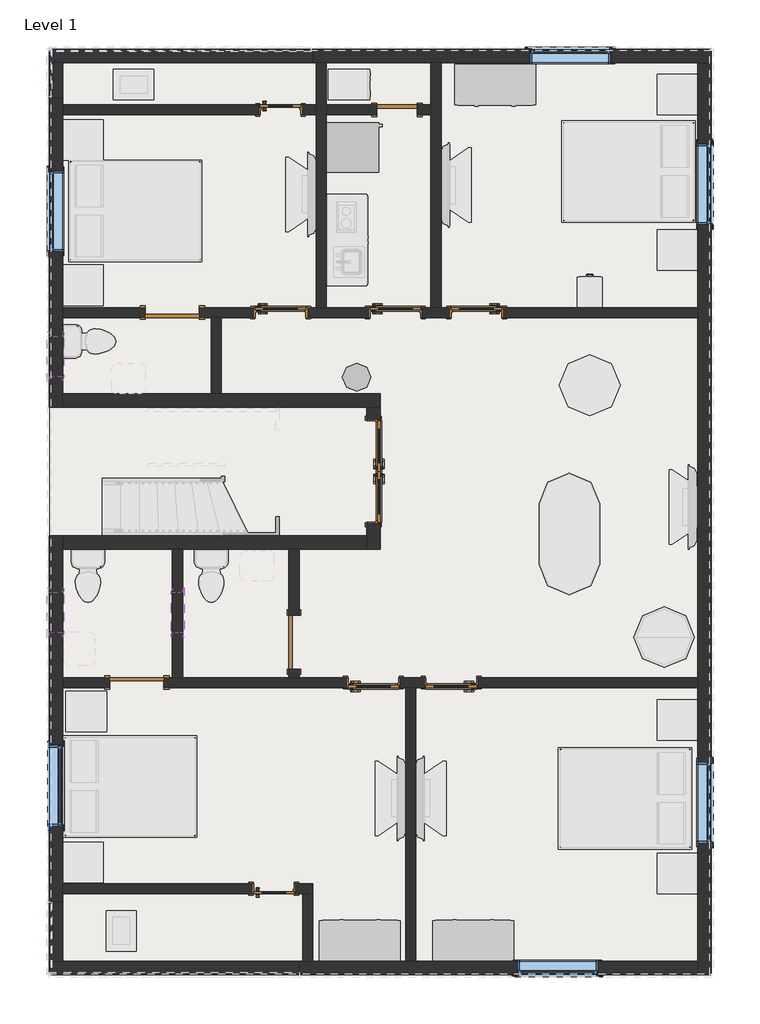
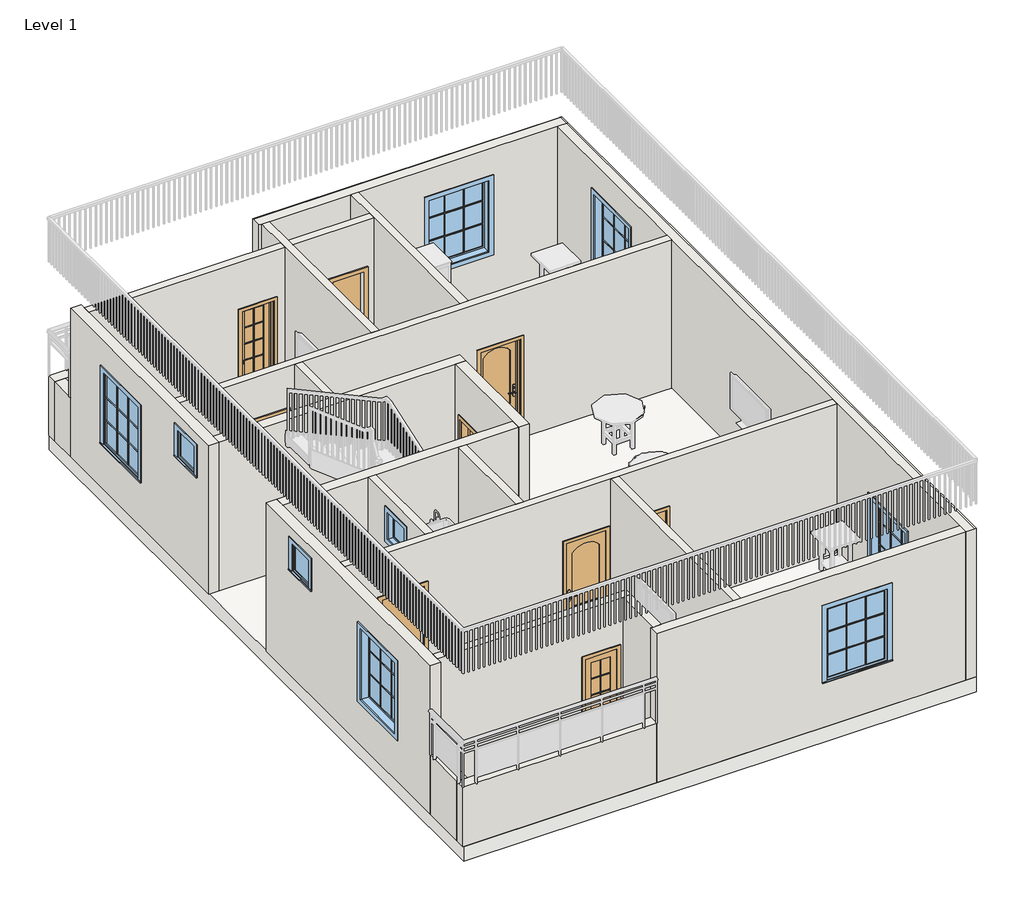
# One storey, part 1 of 7: 24 walls, 12 doors, 9 windows, 1 slab.
"""IFC4 building model written with IfcOpenShell, lengths in millimetres."""

from ifc_helpers import new_model, si_unit, frame, origin, origin_with_axes, place, context, project, spatial, polyline, outline, extrude, faceted_brep, transform, mapped, element, save
from components import door_14b9be53, door_4b146b56, door_b03bd389, door_921d1c85, door_6d64ae12, door_58dae0ba, door_bb092f7c, door_377e7377, window_99fc0ff6, window_2b070d82, window_e41d21a6, window_3d781103

model = new_model("IFC4")

# Units and contexts
model_context = context("Model", 3, world=origin())
ifc_project = project(units=[si_unit("LENGTHUNIT", "METRE", prefix="MILLI")], contexts=[model_context])

# Site, building, storey
site = spatial("IfcSite", under=ifc_project)
building = spatial("IfcBuilding", under=site)
storey = spatial("IfcBuildingStorey", under=building, Name="Level 1", Elevation=0.0)

# Doors
placement = place(None, origin())
door_shape = door_14b9be53(model_context)
element("IfcDoor", 1, ObjectType="30\" x 80\"", at=placement, inside=storey, context=model_context, shape_type="MappedRepresentation", body=[
    mapped(door_shape, transform((-2054.08475, 8491.4589473, 0.0), x_axis=(1.0, 0.0, 0.0), y_axis=(0.0, 1.0, 0.0), z_axis=(0.0, 0.0, 1.0))),
])
element("IfcDoor", 2, ObjectType="30\" x 80\"", at=placement, inside=storey, context=model_context, shape_type="MappedRepresentation", body=[
    mapped(door_shape, transform((-3603.48475, 2922.5089473, 0.0), x_axis=(-1.0, 0.0, 0.0), y_axis=(0.0, -1.0, 0.0), z_axis=(0.0, 0.0, 1.0))),
])
door_2_shape = door_4b146b56(model_context)
element("IfcDoor", 3, ObjectType="30\" x 80\"", at=placement, inside=storey, context=model_context, shape_type="MappedRepresentation", body=[
    mapped(door_2_shape, transform((-2435.08475, 2922.5089473, 0.0), x_axis=(1.0, 0.0, 0.0), y_axis=(0.0, 1.0, 0.0), z_axis=(0.0, 0.0, 1.0))),
])
element("IfcDoor", 4, ObjectType="30\" x 80\"", at=placement, inside=storey, context=model_context, shape_type="MappedRepresentation", body=[
    mapped(door_2_shape, transform((-5000.48475, 8491.4589473, 0.0), x_axis=(-1.0, 0.0, 0.0), y_axis=(0.0, -1.0, 0.0), z_axis=(0.0, 0.0, 1.0))),
])
element("IfcDoor", 5, ObjectType="30\" x 80\"", at=placement, inside=storey, context=model_context, shape_type="MappedRepresentation", body=[
    mapped(door_2_shape, transform((-3273.28475, 8491.4589473, 0.0), x_axis=(-1.0, 0.0, 0.0), y_axis=(0.0, -1.0, 0.0), z_axis=(0.0, 0.0, 1.0))),
])
door_3_shape = door_b03bd389(model_context)
element("IfcDoor", 6, ObjectType="Door-Exterior-Double-Full Glass-Wood_Clad : 60\" x 80\"", at=placement, inside=storey, context=model_context, shape_type="MappedRepresentation", body=[
    mapped(door_3_shape, transform((-3600.30975, 6100.6839473, 0.0), x_axis=(0.0, -1.0, 0.0), y_axis=(1.0, 0.0, 0.0), z_axis=(0.0, 0.0, 1.0))),
])
door_4_shape = door_921d1c85(model_context)
element("IfcDoor", 7, ObjectType="Door-Interior-Single-Full Glass-Wood : 24\" x 80\"", at=placement, inside=storey, context=model_context, shape_type="MappedRepresentation", body=[
    mapped(door_4_shape, transform((-5000.48475, 11539.4589473, 0.0), x_axis=(1.0, 0.0, 0.0), y_axis=(0.0, 1.0, 0.0), z_axis=(0.0, 0.0, 1.0))),
])
door_5_shape = door_6d64ae12(model_context)
element("IfcDoor", 8, ObjectType="Door-Interior-Single-Full Glass-Wood : 24\" x 80\"", at=placement, inside=storey, context=model_context, shape_type="MappedRepresentation", body=[
    mapped(door_5_shape, transform((-5102.08475, -176.2910527, 0.0), x_axis=(1.0, 0.0, 0.0), y_axis=(0.0, 1.0, 0.0), z_axis=(0.0, 0.0, 1.0))),
])
door_6_shape = door_58dae0ba(model_context)
element("IfcDoor", 9, ObjectType="Single-Flush : 24\" x 80\"", at=placement, inside=storey, context=model_context, shape_type="MappedRepresentation", body=[
    mapped(door_6_shape, transform((-3247.88475, 11536.2839473, 0.0), x_axis=(1.0, 0.0, 0.0), y_axis=(0.0, 1.0, 0.0), z_axis=(0.0, 0.0, 1.0))),
])
door_7_shape = door_bb092f7c(model_context)
element("IfcDoor", 10, ObjectType="Single-Flush : 32\" x 84\"", at=placement, inside=storey, context=model_context, shape_type="MappedRepresentation", body=[
    mapped(door_7_shape, transform((-4797.28475, 3535.2839473, 0.0), x_axis=(0.0, -1.0, 0.0), y_axis=(1.0, 0.0, 0.0), z_axis=(0.0, 0.0, 1.0))),
])
element("IfcDoor", 11, ObjectType="Single-Flush : 32\" x 84\"", at=placement, inside=storey, context=model_context, shape_type="MappedRepresentation", body=[
    mapped(door_7_shape, transform((-6626.08475, 8488.2839473, 0.0), x_axis=(1.0, 0.0, 0.0), y_axis=(0.0, 1.0, 0.0), z_axis=(0.0, 0.0, 1.0))),
])
door_8_shape = door_377e7377(model_context)
element("IfcDoor", 12, ObjectType="Single-Flush : 32\" x 84\"", at=placement, inside=storey, context=model_context, shape_type="MappedRepresentation", body=[
    mapped(door_8_shape, transform((-7159.48475, 2925.6839473, 0.0), x_axis=(1.0, 0.0, 0.0), y_axis=(0.0, 1.0, 0.0), z_axis=(0.0, 0.0, 1.0))),
])

# Slab
element("IfcSlab", 13, ObjectType="Generic - 12\"", at=placement, inside=storey, context=model_context, shape_type="SweptSolid", body=[
    extrude(outline(polyline([(-8467.58475, 12450.6839473), (1476.51525, 12450.6839473), (1476.51525, -1468.5160527), (-8467.58475, -1468.5160527), (-8467.58475, 12450.6839473)])), frame((0.0, 0.0, -304.8), z_axis=(0.0, 0.0, 1.0), x_axis=(1.0, 0.0, 0.0)), (0.0, 0.0, 1.0), 304.8),
])

# Walls
element("IfcWall", 14, ObjectType="Generic - 8\"", at=placement, inside=storey, context=model_context, shape_type="Brep", body=[
    faceted_brep([(-8480.28475, 12247.4839473, 0.0), (-8277.08475, 12247.4839473, 0.0), (-4517.88475, 12247.4839473, 0.0), (-4517.88475, 12247.4839473, 1219.2), (-8277.08475, 12247.4839473, 1219.2), (-8480.28475, 12247.4839473, 1219.2), (-8480.28475, 12450.6839473, 0.0), (-8480.28475, 12450.6839473, 1219.2), (-4517.88475, 12450.6839473, 1219.2), (-4517.88475, 12450.6839473, 0.0)], [[[0, 1, 2, 3, 4, 5]], [[6, 7, 8, 9]], [[2, 1, 0, 6, 9]], [[3, 2, 9, 8]], [[5, 4, 3, 8, 7]], [[0, 5, 7, 6]]]),
])
element("IfcWall", 15, ObjectType="Generic - 8\"", at=placement, inside=storey, context=model_context, shape_type="Brep", body=[
    faceted_brep([(1273.31525, 12247.4839473, 0.0), (1273.31525, 8564.4839473, 0.0), (1273.31525, 8412.0839473, 0.0), (1273.31525, 3001.8839473, 0.0), (1273.31525, 2849.4839473, 0.0), (1273.31525, -1265.3160527, 0.0), (1273.31525, -1468.5160527, 0.0), (1273.31525, -1468.5160527, 3048.0), (1273.31525, -1265.3160527, 3048.0), (1273.31525, 2849.4839473, 3048.0), (1273.31525, 3001.8839473, 3048.0), (1273.31525, 8412.0839473, 3048.0), (1273.31525, 8564.4839473, 3048.0), (1273.31525, 12247.4839473, 3048.0), (1273.31525, 512.6839473, 1828.8), (1273.31525, 512.6839473, 304.8), (1273.31525, 1731.8839473, 304.8), (1273.31525, 1731.8839473, 1828.8), (1273.31525, 9809.0839473, 2438.4), (1273.31525, 9809.0839473, 914.4), (1273.31525, 11028.2839473, 914.4), (1273.31525, 11028.2839473, 2438.4), (1476.51525, 12247.4839473, 0.0), (1476.51525, 12247.4839473, 3048.0), (1476.51525, -1468.5160527, 3048.0), (1476.51525, -1468.5160527, 0.0), (1476.51525, 512.6839473, 1828.8), (1476.51525, 1731.8839473, 1828.8), (1476.51525, 1731.8839473, 304.8), (1476.51525, 512.6839473, 304.8), (1476.51525, 9809.0839473, 2438.4), (1476.51525, 11028.2839473, 2438.4), (1476.51525, 11028.2839473, 914.4), (1476.51525, 9809.0839473, 914.4), (1451.11525, 12247.4839473, 3048.0), (1451.11525, -1468.5160527, 3048.0)], [[[0, 1, 2, 3, 4, 5, 6, 7, 8, 9, 10, 11, 12, 13], [14, 15, 16, 17], [18, 19, 20, 21]], [[22, 23, 24, 25], [26, 27, 28, 29], [30, 31, 32, 33]], [[6, 5, 4, 3, 2, 1, 0, 22, 25]], [[0, 13, 34, 23, 22]], [[7, 6, 25, 24, 35]], [[35, 24, 23, 34]], [[13, 12, 11, 10, 9, 8, 7, 35, 34]], [[15, 14, 26, 29]], [[16, 15, 29, 28]], [[17, 16, 28, 27]], [[14, 17, 27, 26]], [[19, 18, 30, 33]], [[20, 19, 33, 32]], [[21, 20, 32, 31]], [[18, 21, 31, 30]]]),
])
element("IfcWall", 16, ObjectType="Generic - 8\"", at=placement, inside=storey, context=model_context, shape_type="Brep", body=[
    faceted_brep([(1273.31525, -1265.3160527, 0.0), (-2968.48475, -1265.3160527, 0.0), (-3120.88475, -1265.3160527, 0.0), (-4517.88475, -1265.3160527, 0.0), (-4670.28475, -1265.3160527, 0.0), (-4721.08475, -1265.3160527, 0.0), (-4721.08475, -1265.3160527, 1219.2), (-4721.08475, -1265.3160527, 3048.0), (-4670.28475, -1265.3160527, 3048.0), (-4517.88475, -1265.3160527, 3048.0), (-3120.88475, -1265.3160527, 3048.0), (-2968.48475, -1265.3160527, 3048.0), (1273.31525, -1265.3160527, 3048.0), (-1444.48475, -1265.3160527, 2438.4), (-1444.48475, -1265.3160527, 914.4), (-225.28475, -1265.3160527, 914.4), (-225.28475, -1265.3160527, 2438.4), (1273.31525, -1468.5160527, 0.0), (1273.31525, -1468.5160527, 3048.0), (-4721.08475, -1468.5160527, 3048.0), (-4721.08475, -1468.5160527, 1219.2), (-4721.08475, -1468.5160527, 0.0), (-1444.48475, -1468.5160527, 2438.4), (-225.28475, -1468.5160527, 2438.4), (-225.28475, -1468.5160527, 914.4), (-1444.48475, -1468.5160527, 914.4)], [[[0, 1, 2, 3, 4, 5, 6, 7, 8, 9, 10, 11, 12], [13, 14, 15, 16]], [[17, 18, 19, 20, 21], [22, 23, 24, 25]], [[5, 4, 3, 2, 1, 0, 17, 21]], [[7, 6, 5, 21, 20, 19]], [[0, 12, 18, 17]], [[12, 11, 10, 9, 8, 7, 19, 18]], [[14, 13, 22, 25]], [[15, 14, 25, 24]], [[16, 15, 24, 23]], [[13, 16, 23, 22]]]),
])
element("IfcWall", 17, ObjectType="Generic - 8\"", at=placement, inside=storey, context=model_context, shape_type="SweptSolid", body=[
    extrude(outline(polyline([(-8277.08475, -376.3160527), (-8277.08475, -1265.3160527), (-8480.28475, -1265.3160527), (-8480.28475, -376.3160527), (-8277.08475, -376.3160527)])), origin_with_axes(), (0.0, 0.0, 1.0), 1219.2),
])
element("IfcWall", 18, ObjectType="Generic - 8\"", at=placement, inside=storey, context=model_context, shape_type="Brep", body=[
    faceted_brep([(-8277.08475, 7065.8839473, 0.0), (-3705.08475, 7065.8839473, 0.0), (-3501.88475, 7065.8839473, 0.0), (-3501.88475, 7065.8839473, 3048.0), (-3705.08475, 7065.8839473, 3048.0), (-6905.48475, 7065.8839473, 3048.0), (-8277.08475, 7065.8839473, 3048.0), (-8277.08475, 7269.0839473, 0.0), (-8277.08475, 7269.0839473, 3048.0), (-6041.88475, 7269.0839473, 3048.0), (-5889.48475, 7269.0839473, 3048.0), (-3501.88475, 7269.0839473, 3048.0), (-3501.88475, 7269.0839473, 0.0), (-5889.48475, 7269.0839473, 0.0), (-6041.88475, 7269.0839473, 0.0)], [[[0, 1, 2, 3, 4, 5, 6]], [[7, 8, 9, 10, 11, 12, 13, 14]], [[2, 1, 0, 7, 14, 13, 12]], [[3, 2, 12, 11]], [[0, 6, 8, 7]], [[6, 5, 4, 3, 11, 10, 9, 8]]]),
])
element("IfcWall", 19, ObjectType="Generic - 8\"", at=placement, inside=storey, context=model_context, shape_type="Brep", body=[
    faceted_brep([(-3705.08475, 7065.8839473, 3048.0), (-3705.08475, 7065.8839473, 0.0), (-3705.08475, 6888.0839473, 0.0), (-3705.08475, 6888.0839473, 2057.4), (-3705.08475, 5313.2839473, 2057.4), (-3705.08475, 5313.2839473, 0.0), (-3705.08475, 5135.4839473, 0.0), (-3705.08475, 4932.2839473, 0.0), (-3705.08475, 4932.2839473, 3048.0), (-3705.08475, 5135.4839473, 3048.0), (-3501.88475, 7065.8839473, 0.0), (-3501.88475, 7065.8839473, 3048.0), (-3501.88475, 4932.2839473, 3048.0), (-3501.88475, 4932.2839473, 0.0), (-3501.88475, 5313.2839473, 0.0), (-3501.88475, 5313.2839473, 2057.4), (-3501.88475, 6888.0839473, 2057.4), (-3501.88475, 6888.0839473, 0.0)], [[[0, 1, 2, 3, 4, 5, 6, 7, 8, 9]], [[10, 11, 12, 13, 14, 15, 16, 17]], [[1, 10, 17, 2]], [[13, 7, 6, 5, 14]], [[1, 0, 11, 10]], [[8, 7, 13, 12]], [[4, 15, 14, 5]], [[15, 4, 3, 16]], [[16, 3, 2, 17]], [[0, 9, 8, 12, 11]]]),
])
element("IfcWall", 20, ObjectType="Generic - 8\"", at=placement, inside=storey, context=model_context, shape_type="Brep", body=[
    faceted_brep([(-3705.08475, 5135.4839473, 0.0), (-8277.08475, 5135.4839473, 0.0), (-8277.08475, 5135.4839473, 3048.0), (-6905.48475, 5135.4839473, 3048.0), (-3705.08475, 5135.4839473, 3048.0), (-3705.08475, 4932.2839473, 0.0), (-3705.08475, 4932.2839473, 3048.0), (-4721.08475, 4932.2839473, 3048.0), (-4873.48475, 4932.2839473, 3048.0), (-6473.68475, 4932.2839473, 3048.0), (-6626.08475, 4932.2839473, 3048.0), (-8277.08475, 4932.2839473, 3048.0), (-8277.08475, 4932.2839473, 0.0), (-6626.08475, 4932.2839473, 0.0), (-6473.68475, 4932.2839473, 0.0), (-4873.48475, 4932.2839473, 0.0), (-4721.08475, 4932.2839473, 0.0)], [[[0, 1, 2, 3, 4]], [[5, 6, 7, 8, 9, 10, 11, 12, 13, 14, 15, 16]], [[1, 0, 5, 16, 15, 14, 13, 12]], [[0, 4, 6, 5]], [[2, 1, 12, 11]], [[4, 3, 2, 11, 10, 9, 8, 7, 6]]]),
])
element("IfcWall", 21, ObjectType="Generic - 8\"", at=placement, inside=storey, context=model_context, shape_type="Brep", body=[
    faceted_brep([(-4517.88475, 12247.4839473, 0.0), (-4467.08475, 12247.4839473, 0.0), (-4314.68475, 12247.4839473, 0.0), (-2739.88475, 12247.4839473, 0.0), (-2587.48475, 12247.4839473, 0.0), (1273.31525, 12247.4839473, 0.0), (1476.51525, 12247.4839473, 0.0), (1476.51525, 12247.4839473, 3048.0), (1451.11525, 12247.4839473, 3048.0), (1273.31525, 12247.4839473, 3048.0), (-2587.48475, 12247.4839473, 3048.0), (-2739.88475, 12247.4839473, 3048.0), (-4314.68475, 12247.4839473, 3048.0), (-4467.08475, 12247.4839473, 3048.0), (-4517.88475, 12247.4839473, 3048.0), (-4517.88475, 12247.4839473, 1219.2), (-34.78475, 12247.4839473, 2438.4), (-34.78475, 12247.4839473, 914.4), (-1253.98475, 12247.4839473, 914.4), (-1253.98475, 12247.4839473, 2438.4), (-4517.88475, 12450.6839473, 0.0), (-4517.88475, 12450.6839473, 1219.2), (-4517.88475, 12450.6839473, 3048.0), (1451.11525, 12450.6839473, 3048.0), (1476.51525, 12450.6839473, 3048.0), (1476.51525, 12450.6839473, 0.0), (-34.78475, 12450.6839473, 2438.4), (-1253.98475, 12450.6839473, 2438.4), (-1253.98475, 12450.6839473, 914.4), (-34.78475, 12450.6839473, 914.4), (-4517.88475, 12437.9839473, 3048.0), (1476.51525, 12437.9839473, 3048.0), (1451.11525, 12437.9839473, 3048.0)], [[[0, 1, 2, 3, 4, 5, 6, 7, 8, 9, 10, 11, 12, 13, 14, 15], [16, 17, 18, 19]], [[20, 21, 22, 23, 24, 25], [26, 27, 28, 29]], [[6, 5, 4, 3, 2, 1, 0, 20, 25]], [[0, 15, 14, 30, 22, 21, 20]], [[7, 6, 25, 24, 31]], [[8, 7, 31, 32]], [[23, 22, 30, 32]], [[31, 24, 23, 32]], [[14, 13, 12, 11, 10, 9, 8, 32, 30]], [[17, 16, 26, 29]], [[18, 17, 29, 28]], [[19, 18, 28, 27]], [[16, 19, 27, 26]]]),
])
element("IfcWall", 22, ObjectType="Generic - 8\"", at=placement, inside=storey, context=model_context, shape_type="SweptSolid", body=[
    extrude(outline(polyline([(-8277.08475, 12247.4839473), (-8277.08475, 11714.0839473), (-8480.28475, 11714.0839473), (-8480.28475, 12247.4839473), (-8277.08475, 12247.4839473)])), origin_with_axes(), (0.0, 0.0, 1.0), 1219.2),
])
element("IfcWall", 23, ObjectType="Generic - 8\"", at=placement, inside=storey, context=model_context, shape_type="Brep", body=[
    faceted_brep([(-8277.08475, -376.3160527, 0.0), (-8277.08475, -249.3160527, 0.0), (-8277.08475, -96.9160527, 0.0), (-8277.08475, 2849.4839473, 0.0), (-8277.08475, 3001.8839473, 0.0), (-8277.08475, 4932.2839473, 0.0), (-8277.08475, 5135.4839473, 0.0), (-8277.08475, 5135.4839473, 3048.0), (-8277.08475, 4932.2839473, 3048.0), (-8277.08475, 3001.8839473, 3048.0), (-8277.08475, 2849.4839473, 3048.0), (-8277.08475, -96.9160527, 3048.0), (-8277.08475, -249.3160527, 3048.0), (-8277.08475, -376.3160527, 3048.0), (-8277.08475, -376.3160527, 1219.2), (-8277.08475, 1985.8839473, 2438.4), (-8277.08475, 1985.8839473, 914.4), (-8277.08475, 766.6839473, 914.4), (-8277.08475, 766.6839473, 2438.4), (-8277.08475, 4284.5839473, 2768.6), (-8277.08475, 4284.5839473, 2159.0), (-8277.08475, 3674.9839473, 2159.0), (-8277.08475, 3674.9839473, 2768.6), (-8480.28475, -376.3160527, 0.0), (-8480.28475, -376.3160527, 1219.2), (-8480.28475, -376.3160527, 3048.0), (-8480.28475, 5135.4839473, 3048.0), (-8480.28475, 5135.4839473, 0.0), (-8480.28475, 1985.8839473, 2438.4), (-8480.28475, 766.6839473, 2438.4), (-8480.28475, 766.6839473, 914.4), (-8480.28475, 1985.8839473, 914.4), (-8480.28475, 4284.5839473, 2768.6), (-8480.28475, 3674.9839473, 2768.6), (-8480.28475, 3674.9839473, 2159.0), (-8480.28475, 4284.5839473, 2159.0)], [[[0, 1, 2, 3, 4, 5, 6, 7, 8, 9, 10, 11, 12, 13, 14], [15, 16, 17, 18], [19, 20, 21, 22]], [[23, 24, 25, 26, 27], [28, 29, 30, 31], [32, 33, 34, 35]], [[6, 5, 4, 3, 2, 1, 0, 23, 27]], [[0, 14, 13, 25, 24, 23]], [[7, 6, 27, 26]], [[13, 12, 11, 10, 9, 8, 7, 26, 25]], [[16, 15, 28, 31]], [[17, 16, 31, 30]], [[18, 17, 30, 29]], [[15, 18, 29, 28]], [[20, 19, 32, 35]], [[21, 20, 35, 34]], [[22, 21, 34, 33]], [[19, 22, 33, 32]]]),
])
element("IfcWall", 24, ObjectType="Generic - 8\"", at=placement, inside=storey, context=model_context, shape_type="Brep", body=[
    faceted_brep([(-4721.08475, -1265.3160527, 0.0), (-8277.08475, -1265.3160527, 0.0), (-8480.28475, -1265.3160527, 0.0), (-8480.28475, -1265.3160527, 1219.2), (-8277.08475, -1265.3160527, 1219.2), (-4721.08475, -1265.3160527, 1219.2), (-4721.08475, -1468.5160527, 0.0), (-4721.08475, -1468.5160527, 1219.2), (-8480.28475, -1468.5160527, 1219.2), (-8480.28475, -1468.5160527, 0.0)], [[[0, 1, 2, 3, 4, 5]], [[6, 7, 8, 9]], [[2, 1, 0, 6, 9]], [[5, 4, 3, 8, 7]], [[0, 5, 7, 6]], [[3, 2, 9, 8]]]),
])
element("IfcWall", 25, ObjectType="Generic - 8\"", at=placement, inside=storey, context=model_context, shape_type="Brep", body=[
    faceted_brep([(-8277.08475, 7065.8839473, 0.0), (-8277.08475, 7269.0839473, 0.0), (-8277.08475, 8412.0839473, 0.0), (-8277.08475, 8564.4839473, 0.0), (-8277.08475, 11460.0839473, 0.0), (-8277.08475, 11612.4839473, 0.0), (-8277.08475, 11714.0839473, 0.0), (-8277.08475, 11714.0839473, 1219.2), (-8277.08475, 11714.0839473, 3048.0), (-8277.08475, 11612.4839473, 3048.0), (-8277.08475, 11460.0839473, 3048.0), (-8277.08475, 8564.4839473, 3048.0), (-8277.08475, 8412.0839473, 3048.0), (-8277.08475, 7269.0839473, 3048.0), (-8277.08475, 7065.8839473, 3048.0), (-8277.08475, 10621.8839473, 2438.4), (-8277.08475, 10621.8839473, 914.4), (-8277.08475, 9402.6839473, 914.4), (-8277.08475, 9402.6839473, 2438.4), (-8277.08475, 8132.6839473, 2768.6), (-8277.08475, 8132.6839473, 2159.0), (-8277.08475, 7523.0839473, 2159.0), (-8277.08475, 7523.0839473, 2768.6), (-8480.28475, 7065.8839473, 0.0), (-8480.28475, 7065.8839473, 3048.0), (-8480.28475, 11714.0839473, 3048.0), (-8480.28475, 11714.0839473, 1219.2), (-8480.28475, 11714.0839473, 0.0), (-8480.28475, 10621.8839473, 2438.4), (-8480.28475, 9402.6839473, 2438.4), (-8480.28475, 9402.6839473, 914.4), (-8480.28475, 10621.8839473, 914.4), (-8480.28475, 8132.6839473, 2768.6), (-8480.28475, 7523.0839473, 2768.6), (-8480.28475, 7523.0839473, 2159.0), (-8480.28475, 8132.6839473, 2159.0)], [[[0, 1, 2, 3, 4, 5, 6, 7, 8, 9, 10, 11, 12, 13, 14], [15, 16, 17, 18], [19, 20, 21, 22]], [[23, 24, 25, 26, 27], [28, 29, 30, 31], [32, 33, 34, 35]], [[6, 5, 4, 3, 2, 1, 0, 23, 27]], [[8, 7, 6, 27, 26, 25]], [[0, 14, 24, 23]], [[14, 13, 12, 11, 10, 9, 8, 25, 24]], [[16, 15, 28, 31]], [[17, 16, 31, 30]], [[18, 17, 30, 29]], [[15, 18, 29, 28]], [[20, 19, 32, 35]], [[21, 20, 35, 34]], [[22, 21, 34, 33]], [[19, 22, 33, 32]]]),
])
element("IfcWall", 26, ObjectType="INNER WALL", at=placement, inside=storey, context=model_context, shape_type="Brep", body=[
    faceted_brep([(-8277.08475, -249.3160527, 3048.0), (-8277.08475, -249.3160527, 0.0), (-5432.28475, -249.3160527, 0.0), (-5432.28475, -249.3160527, 2057.4), (-4771.88475, -249.3160527, 2057.4), (-4771.88475, -249.3160527, 0.0), (-4670.28475, -249.3160527, 0.0), (-4517.88475, -249.3160527, 0.0), (-4517.88475, -249.3160527, 3048.0), (-4670.28475, -249.3160527, 3048.0), (-8277.08475, -96.9160527, 0.0), (-8277.08475, -96.9160527, 3048.0), (-4517.88475, -96.9160527, 3048.0), (-4517.88475, -96.9160527, 0.0), (-4771.88475, -96.9160527, 0.0), (-4771.88475, -96.9160527, 2057.4), (-5432.28475, -96.9160527, 2057.4), (-5432.28475, -96.9160527, 0.0)], [[[0, 1, 2, 3, 4, 5, 6, 7, 8, 9]], [[10, 11, 12, 13, 14, 15, 16, 17]], [[1, 10, 17, 2]], [[13, 7, 6, 5, 14]], [[1, 0, 11, 10]], [[8, 7, 13, 12]], [[4, 15, 14, 5]], [[15, 4, 3, 16]], [[16, 3, 2, 17]], [[0, 9, 8, 12, 11]]]),
])
element("IfcWall", 27, ObjectType="INNER WALL", at=placement, inside=storey, context=model_context, shape_type="SweptSolid", body=[
    extrude(outline(polyline([(-4670.28475, -1265.3160527), (-4670.28475, -249.3160527), (-4517.88475, -249.3160527), (-4517.88475, -1265.3160527), (-4670.28475, -1265.3160527)])), origin_with_axes(), (0.0, 0.0, 1.0), 3048.0),
])
element("IfcWall", 28, ObjectType="INNER WALL", at=placement, inside=storey, context=model_context, shape_type="SweptSolid", body=[
    extrude(outline(polyline([(-2968.48475, 2849.4839473), (-2968.48475, -1265.3160527), (-3120.88475, -1265.3160527), (-3120.88475, 2849.4839473), (-2968.48475, 2849.4839473)])), origin_with_axes(), (0.0, 0.0, 1.0), 3048.0),
])
element("IfcWall", 29, ObjectType="INNER WALL", at=placement, inside=storey, context=model_context, shape_type="Brep", body=[
    faceted_brep([(-8277.08475, 3001.8839473, 0.0), (-8277.08475, 3001.8839473, 3048.0), (-6626.08475, 3001.8839473, 3048.0), (-6473.68475, 3001.8839473, 3048.0), (-4873.48475, 3001.8839473, 3048.0), (-4721.08475, 3001.8839473, 3048.0), (1273.31525, 3001.8839473, 3048.0), (1273.31525, 3001.8839473, 0.0), (-2028.68475, 3001.8839473, 0.0), (-2028.68475, 3001.8839473, 2057.4), (-2841.48475, 3001.8839473, 2057.4), (-2841.48475, 3001.8839473, 0.0), (-3197.08475, 3001.8839473, 0.0), (-3197.08475, 3001.8839473, 2057.4), (-4009.88475, 3001.8839473, 2057.4), (-4009.88475, 3001.8839473, 0.0), (-4721.08475, 3001.8839473, 0.0), (-4873.48475, 3001.8839473, 0.0), (-6473.68475, 3001.8839473, 0.0), (-6626.08475, 3001.8839473, 0.0), (-6753.08475, 3001.8839473, 0.0), (-6753.08475, 3001.8839473, 2133.6), (-7565.88475, 3001.8839473, 2133.6), (-7565.88475, 3001.8839473, 0.0), (-8277.08475, 2849.4839473, 3048.0), (-8277.08475, 2849.4839473, 0.0), (-7565.88475, 2849.4839473, 0.0), (-7565.88475, 2849.4839473, 2133.6), (-6753.08475, 2849.4839473, 2133.6), (-6753.08475, 2849.4839473, 0.0), (-4009.88475, 2849.4839473, 0.0), (-4009.88475, 2849.4839473, 2057.4), (-3197.08475, 2849.4839473, 2057.4), (-3197.08475, 2849.4839473, 0.0), (-3120.88475, 2849.4839473, 0.0), (-2968.48475, 2849.4839473, 0.0), (-2841.48475, 2849.4839473, 0.0), (-2841.48475, 2849.4839473, 2057.4), (-2028.68475, 2849.4839473, 2057.4), (-2028.68475, 2849.4839473, 0.0), (1273.31525, 2849.4839473, 0.0), (1273.31525, 2849.4839473, 3048.0), (-2968.48475, 2849.4839473, 3048.0), (-3120.88475, 2849.4839473, 3048.0)], [[[0, 1, 2, 3, 4, 5, 6, 7, 8, 9, 10, 11, 12, 13, 14, 15, 16, 17, 18, 19, 20, 21, 22, 23]], [[24, 25, 26, 27, 28, 29, 30, 31, 32, 33, 34, 35, 36, 37, 38, 39, 40, 41, 42, 43]], [[25, 0, 23, 26]], [[7, 40, 39, 8]], [[29, 20, 19, 18, 17, 16, 15, 30]], [[11, 36, 35, 34, 33, 12]], [[1, 0, 25, 24]], [[7, 6, 41, 40]], [[21, 20, 29, 28]], [[22, 21, 28, 27]], [[23, 22, 27, 26]], [[38, 9, 8, 39]], [[9, 38, 37, 10]], [[10, 37, 36, 11]], [[14, 31, 30, 15]], [[31, 14, 13, 32]], [[32, 13, 12, 33]], [[6, 5, 4, 3, 2, 1, 24, 43, 42, 41]]]),
])
element("IfcWall", 30, ObjectType="INNER WALL", at=placement, inside=storey, context=model_context, shape_type="SweptSolid", body=[
    extrude(outline(polyline([(3048.0, -8277.08475), (0.0, -8277.08475), (0.0, -5330.68475), (2057.4, -5330.68475), (2057.4, -4670.28475), (0.0, -4670.28475), (0.0, -4467.08475), (3048.0, -4467.08475), (3048.0, -8277.08475)])), frame((0.0, 11460.0839473, 0.0), z_axis=(0.0, 1.0, 0.0), x_axis=(0.0, 0.0, 1.0)), (0.0, 0.0, 1.0), 152.4),
])
element("IfcWall", 31, ObjectType="INNER WALL", at=placement, inside=storey, context=model_context, shape_type="Brep", body=[
    faceted_brep([(-4314.68475, 8564.4839473, 0.0), (-4314.68475, 11460.0839473, 0.0), (-4314.68475, 11612.4839473, 0.0), (-4314.68475, 12247.4839473, 0.0), (-4314.68475, 12247.4839473, 3048.0), (-4314.68475, 11612.4839473, 3048.0), (-4314.68475, 11460.0839473, 3048.0), (-4314.68475, 8564.4839473, 3048.0), (-4467.08475, 8564.4839473, 0.0), (-4467.08475, 8564.4839473, 3048.0), (-4467.08475, 11460.0839473, 3048.0), (-4467.08475, 11612.4839473, 3048.0), (-4467.08475, 12247.4839473, 3048.0), (-4467.08475, 12247.4839473, 0.0), (-4467.08475, 11612.4839473, 0.0), (-4467.08475, 11460.0839473, 0.0)], [[[0, 1, 2, 3, 4, 5, 6, 7]], [[8, 9, 10, 11, 12, 13, 14, 15]], [[3, 2, 1, 0, 8, 15, 14, 13]], [[4, 3, 13, 12]], [[0, 7, 9, 8]], [[7, 6, 5, 4, 12, 11, 10, 9]]]),
])
element("IfcWall", 32, ObjectType="INNER WALL", at=placement, inside=storey, context=model_context, shape_type="Brep", body=[
    faceted_brep([(-2739.88475, 12247.4839473, 0.0), (-2739.88475, 11612.4839473, 0.0), (-2739.88475, 11460.0839473, 0.0), (-2739.88475, 8564.4839473, 0.0), (-2739.88475, 8564.4839473, 3048.0), (-2739.88475, 11460.0839473, 3048.0), (-2739.88475, 11612.4839473, 3048.0), (-2739.88475, 12247.4839473, 3048.0), (-2587.48475, 12247.4839473, 0.0), (-2587.48475, 12247.4839473, 3048.0), (-2587.48475, 8564.4839473, 3048.0), (-2587.48475, 8564.4839473, 0.0)], [[[0, 1, 2, 3, 4, 5, 6, 7]], [[8, 9, 10, 11]], [[3, 2, 1, 0, 8, 11]], [[0, 7, 9, 8]], [[4, 3, 11, 10]], [[7, 6, 5, 4, 10, 9]]]),
])
element("IfcWall", 33, ObjectType="INNER WALL", at=placement, inside=storey, context=model_context, shape_type="Brep", body=[
    faceted_brep([(1273.31525, 8412.0839473, 0.0), (1273.31525, 8412.0839473, 3048.0), (-5889.48475, 8412.0839473, 3048.0), (-6041.88475, 8412.0839473, 3048.0), (-8277.08475, 8412.0839473, 3048.0), (-8277.08475, 8412.0839473, 0.0), (-7032.48475, 8412.0839473, 0.0), (-7032.48475, 8412.0839473, 2133.6), (-6219.68475, 8412.0839473, 2133.6), (-6219.68475, 8412.0839473, 0.0), (-6041.88475, 8412.0839473, 0.0), (-5889.48475, 8412.0839473, 0.0), (-5406.88475, 8412.0839473, 0.0), (-5406.88475, 8412.0839473, 2057.4), (-4594.08475, 8412.0839473, 2057.4), (-4594.08475, 8412.0839473, 0.0), (-3679.68475, 8412.0839473, 0.0), (-3679.68475, 8412.0839473, 2057.4), (-2866.88475, 8412.0839473, 2057.4), (-2866.88475, 8412.0839473, 0.0), (-2460.48475, 8412.0839473, 0.0), (-2460.48475, 8412.0839473, 2057.4), (-1647.68475, 8412.0839473, 2057.4), (-1647.68475, 8412.0839473, 0.0), (1273.31525, 8564.4839473, 3048.0), (1273.31525, 8564.4839473, 0.0), (-1647.68475, 8564.4839473, 0.0), (-1647.68475, 8564.4839473, 2057.4), (-2460.48475, 8564.4839473, 2057.4), (-2460.48475, 8564.4839473, 0.0), (-2587.48475, 8564.4839473, 0.0), (-2739.88475, 8564.4839473, 0.0), (-2866.88475, 8564.4839473, 0.0), (-2866.88475, 8564.4839473, 2057.4), (-3679.68475, 8564.4839473, 2057.4), (-3679.68475, 8564.4839473, 0.0), (-4314.68475, 8564.4839473, 0.0), (-4467.08475, 8564.4839473, 0.0), (-4594.08475, 8564.4839473, 0.0), (-4594.08475, 8564.4839473, 2057.4), (-5406.88475, 8564.4839473, 2057.4), (-5406.88475, 8564.4839473, 0.0), (-6219.68475, 8564.4839473, 0.0), (-6219.68475, 8564.4839473, 2133.6), (-7032.48475, 8564.4839473, 2133.6), (-7032.48475, 8564.4839473, 0.0), (-8277.08475, 8564.4839473, 0.0), (-8277.08475, 8564.4839473, 3048.0), (-4467.08475, 8564.4839473, 3048.0), (-4314.68475, 8564.4839473, 3048.0), (-2739.88475, 8564.4839473, 3048.0), (-2587.48475, 8564.4839473, 3048.0)], [[[0, 1, 2, 3, 4, 5, 6, 7, 8, 9, 10, 11, 12, 13, 14, 15, 16, 17, 18, 19, 20, 21, 22, 23]], [[24, 25, 26, 27, 28, 29, 30, 31, 32, 33, 34, 35, 36, 37, 38, 39, 40, 41, 42, 43, 44, 45, 46, 47, 48, 49, 50, 51]], [[25, 0, 23, 26]], [[5, 46, 45, 6]], [[9, 42, 41, 12, 11, 10]], [[29, 20, 19, 32, 31, 30]], [[15, 38, 37, 36, 35, 16]], [[1, 0, 25, 24]], [[5, 4, 47, 46]], [[43, 42, 9, 8]], [[44, 43, 8, 7]], [[45, 44, 7, 6]], [[22, 27, 26, 23]], [[27, 22, 21, 28]], [[28, 21, 20, 29]], [[40, 13, 12, 41]], [[13, 40, 39, 14]], [[14, 39, 38, 15]], [[34, 17, 16, 35]], [[17, 34, 33, 18]], [[18, 33, 32, 19]], [[4, 3, 2, 1, 24, 51, 50, 49, 48, 47]]]),
])
element("IfcWall", 34, ObjectType="INNER WALL", at=placement, inside=storey, context=model_context, shape_type="SweptSolid", body=[
    extrude(outline(polyline([(-5889.48475, 8412.0839473), (-5889.48475, 7269.0839473), (-6041.88475, 7269.0839473), (-6041.88475, 8412.0839473), (-5889.48475, 8412.0839473)])), origin_with_axes(), (0.0, 0.0, 1.0), 3048.0),
])
element("IfcWall", 35, ObjectType="INNER WALL", at=placement, inside=storey, context=model_context, shape_type="SweptSolid", body=[
    extrude(outline(polyline([(2032.0, -2943.08475), (0.0, -2943.08475), (0.0, -2739.88475), (3048.0, -2739.88475), (3048.0, -4314.68475), (0.0, -4314.68475), (0.0, -3552.68475), (2032.0, -3552.68475), (2032.0, -2943.08475)])), frame((0.0, 11460.0839473, 0.0), z_axis=(0.0, 1.0, 0.0), x_axis=(0.0, 0.0, 1.0)), (0.0, 0.0, 1.0), 152.4),
])
element("IfcWall", 36, ObjectType="INNER WALL", at=placement, inside=storey, context=model_context, shape_type="SweptSolid", body=[
    extrude(outline(polyline([(4932.2839473, 0.0), (3001.8839473, 0.0), (3001.8839473, 3048.0), (4932.2839473, 3048.0), (4932.2839473, 0.0)]), holes=[polyline([(3674.9839473, 2768.6), (3674.9839473, 2159.0), (4284.5839473, 2159.0), (4284.5839473, 2768.6), (3674.9839473, 2768.6)])]), frame((-6626.08475, 0.0, 0.0), z_axis=(1.0, 0.0, 0.0), x_axis=(0.0, 1.0, 0.0)), (0.0, 0.0, 1.0), 152.4),
])
element("IfcWall", 37, ObjectType="INNER WALL", at=placement, inside=storey, context=model_context, shape_type="SweptSolid", body=[
    extrude(outline(polyline([(3128.8839473, 2133.6), (3128.8839473, 0.0), (3001.8839473, 0.0), (3001.8839473, 3048.0), (4932.2839473, 3048.0), (4932.2839473, 0.0), (3941.6839473, 0.0), (3941.6839473, 2133.6), (3128.8839473, 2133.6)])), frame((-4873.48475, 0.0, 0.0), z_axis=(1.0, 0.0, 0.0), x_axis=(0.0, 1.0, 0.0)), (0.0, 0.0, 1.0), 152.4),
])

# Windows
window_shape = window_99fc0ff6(model_context)
element("IfcWindow", 38, ObjectType="Casement 3x3 with Trim : 48\" x 60\"", at=placement, inside=storey, context=model_context, shape_type="MappedRepresentation", body=[
    mapped(window_shape, transform((-834.88475, -1366.9160527, 609.6), x_axis=(-1.0, 0.0, 0.0), y_axis=(0.0, -1.0, 0.0), z_axis=(0.0, 0.0, 1.0))),
])
element("IfcWindow", 39, ObjectType="Casement 3x3 with Trim : 48\" x 60\"", at=placement, inside=storey, context=model_context, shape_type="MappedRepresentation", body=[
    mapped(window_shape, transform((1374.91525, 1122.2839473, 0.0), x_axis=(0.0, -1.0, 0.0), y_axis=(1.0, 0.0, 0.0), z_axis=(0.0, 0.0, 1.0))),
])
element("IfcWindow", 40, ObjectType="Casement 3x3 with Trim : 48\" x 60\"", at=placement, inside=storey, context=model_context, shape_type="MappedRepresentation", body=[
    mapped(window_shape, transform((-8378.68475, 10012.2839473, 609.6), x_axis=(0.0, 1.0, 0.0), y_axis=(-1.0, 0.0, 0.0), z_axis=(0.0, 0.0, 1.0))),
])
element("IfcWindow", 41, ObjectType="Casement 3x3 with Trim : 48\" x 60\"", at=placement, inside=storey, context=model_context, shape_type="MappedRepresentation", body=[
    mapped(window_shape, transform((-644.38475, 12349.0839473, 609.6), x_axis=(1.0, 0.0, 0.0), y_axis=(0.0, 1.0, 0.0), z_axis=(0.0, 0.0, 1.0))),
])
element("IfcWindow", 42, ObjectType="Casement 3x3 with Trim : 48\" x 60\"", at=placement, inside=storey, context=model_context, shape_type="MappedRepresentation", body=[
    mapped(window_shape, transform((1374.91525, 10418.6839473, 609.6), x_axis=(0.0, -1.0, 0.0), y_axis=(1.0, 0.0, 0.0), z_axis=(0.0, 0.0, 1.0))),
])
window_2_shape = window_2b070d82(model_context)
element("IfcWindow", 43, ObjectType="Casement 3x3 with Trim : 48\" x 60\"", at=placement, inside=storey, context=model_context, shape_type="MappedRepresentation", body=[
    mapped(window_2_shape, transform((-8378.68475, 1376.2839473, 609.6), x_axis=(0.0, 1.0, 0.0), y_axis=(-1.0, 0.0, 0.0), z_axis=(0.0, 0.0, 1.0))),
])
window_3_shape = window_e41d21a6(model_context)
element("IfcWindow", 44, ObjectType="Transom with Trim : 24\" x 24\"", at=placement, inside=storey, context=model_context, shape_type="MappedRepresentation", body=[
    mapped(window_3_shape, transform((-8378.68475, 4017.8839473, 0.0), x_axis=(0.0, 1.0, 0.0), y_axis=(-1.0, 0.0, 0.0), z_axis=(0.0, 0.0, 1.0))),
])
element("IfcWindow", 45, ObjectType="Transom with Trim : 24\" x 24\"", at=placement, inside=storey, context=model_context, shape_type="MappedRepresentation", body=[
    mapped(window_3_shape, transform((-8378.68475, 7865.9839473, 0.0), x_axis=(0.0, 1.0, 0.0), y_axis=(-1.0, 0.0, 0.0), z_axis=(0.0, 0.0, 1.0))),
])
window_4_shape = window_3d781103(model_context)
element("IfcWindow", 46, ObjectType="Transom with Trim : 24\" x 24\"", at=placement, inside=storey, context=model_context, shape_type="MappedRepresentation", body=[
    mapped(window_4_shape, transform((-6549.88475, 3941.6839473, 0.0), x_axis=(0.0, -1.0, 0.0), y_axis=(1.0, 0.0, 0.0), z_axis=(0.0, 0.0, 1.0))),
])

save(model, "model.ifc")

# Revit data of these elements
# Type "30\" x 80\""
#   Type Mark = "9"
#   Assembly Code = "B2030100"
#   Analytic Construction = "French door, wood frame with single glass"
#   Threshold Offset [instance default] = 0' - 0 1/2"
#   Thickness = 0' - 1 3/8"
#   Thermal Resistance (R) = 1.0696 (h·ft²·°F)/BTU
#   Swing Angle [instance default] = 90.00°
#   Stiles = 0' - 4 3/4"
#   Rough Width = 2' - 8"
#   Rough Height = 6' - 9"
#   Radius = 1' - 1.00625"
#   Lock Rail = 0' - 7 1/8"
#   Height = 6' - 8"
#   Width = 2' - 6"
#   Heat Transfer Coefficient (U) = 0.9350 BTU/(h·ft²·°F)
#   Door Offset [instance default] = 0' - 0"
#   Bottom Rail = 0' - 9 1/2"
#   Threshold [instance default] = yes
#   Function = 1
#   Exterior Trim [instance default] = yes
#   Trim Material = Cherry
#   Threshold Material = Cherry
#   Panel Material = Cherry
#   Glazing = Glass
#   Frame Material = Cherry
#   Door Handle Material = Aluminum
#   Visual Light Transmittance = 0
#   Solar Heat Gain Coefficient = 0
#   Wall Closure = (empty or 0)
#   Construction Type = (empty or 0)
# Type "Door-Exterior-Double-Full Glass-Wood_Clad : 60\" x 80\""
#   Type Mark = "8"
#   Assembly Code = "B2030100"
#   Analytic Construction = "French door, wood frame with double glass"
#   Top Rail = 0' - 4 11/16"
#   Threshold Offset [instance default] = 0' - 0 1/2"
#   Thickness = 0' - 1 3/8"
#   Thermal Resistance (R) = 1.9158 (h·ft²·°F)/BTU
#   Swing Angle [instance default] = 90.00°
#   Stiles = 0' - 4 3/4"
#   Rough Width = 5' - 2"
#   Rough Height = 6' - 9"
#   Panel Width = 2' - 6"
#   Door Offset [instance default] = 0' - 0"
#   Height = 6' - 8"
#   Width = 5' - 0"
#   Heat Transfer Coefficient (U) = 0.5220 BTU/(h·ft²·°F)
#   Bottom Rail = 0' - 9 1/8"
#   Exterior Trim [instance default] = yes
#   Threshold [instance default] = yes
#   Show Grill [instance default] = yes
#   Function = 1
#   Trim Material = Cherry
#   Threshold Material = Cherry
#   Panel Material = Cherry
#   Glazing = Glass
#   Frame Material = Cherry
#   Door Handle Material = Aluminum
#   Visual Light Transmittance = 0
#   Solar Heat Gain Coefficient = 0
#   Wall Closure = (empty or 0)
#   Construction Type = (empty or 0)
# Type "Door-Interior-Single-Full Glass-Wood : 24\" x 80\""
#   Type Mark = "10"
#   Assembly Code = "C1020300"
#   Analytic Construction = "Wood frame with single clear glass"
#   Top Rail = 0' - 4 11/16"
#   Thickness = 0' - 1 3/8"
#   Thermal Resistance (R) = 1.0102 (h·ft²·°F)/BTU
#   Swing Angle [instance default] = 90.00°
#   Stiles = 0' - 4 3/4"
#   Rough Width = 2' - 2"
#   Rough Height = 6' - 9"
#   Height = 6' - 8"
#   Width = 2' - 0"
#   Heat Transfer Coefficient (U) = 0.9900 BTU/(h·ft²·°F)
#   Bottom Rail = 0' - 9 1/8"
#   Show Grill [instance default] = yes
#   Trim Material = Cherry
#   Panel Material = Cherry
#   Frame Material = Cherry
#   Door Handle Material = Aluminum
#   Visual Light Transmittance = 0
#   Solar Heat Gain Coefficient = 0
#   Wall Closure = (empty or 0)
#   Function = (empty or 0)
# Type "Single-Flush : 24\" x 80\""
#   Type Mark = "5"
#   Construction Type Id = "MDOOR"
#   Assembly Code = "C1020"
#   Analytic Construction = "Metal"
#   Thickness = 0' - 2"
#   Heat Transfer Coefficient (U) = 0.651978 BTU/(h·ft²·°F)
#   Height = 6' - 8"
#   Trim Projection Ext = 0' - 1"
#   Trim Projection Int = 0' - 1"
#   Trim Width = 0' - 3"
#   Width = 2' - 0"
#   Define Thermal Properties by = 1
#   Door Material = Door - Panel
#   Frame Material = Door - Frame
#   Visual Light Transmittance = 0
#   Solar Heat Gain Coefficient = 0
#   Function = (empty or 0)
#   Wall Closure = (empty or 0)
# Type "Single-Flush : 32\" x 84\""
#   Type Mark = "3"
#   Construction Type Id = "MDOOR"
#   Assembly Code = "C1020"
#   Analytic Construction = "Metal"
#   Thickness = 0' - 2"
#   Heat Transfer Coefficient (U) = 0.651978 BTU/(h·ft²·°F)
#   Height = 7' - 0"
#   Trim Projection Ext = 0' - 1"
#   Trim Projection Int = 0' - 1"
#   Trim Width = 0' - 3"
#   Width = 2' - 8"
#   Define Thermal Properties by = 1
#   Door Material = Door - Panel
#   Frame Material = Door - Frame
#   Visual Light Transmittance = 0
#   Solar Heat Gain Coefficient = 0
#   Function = (empty or 0)
#   Wall Closure = (empty or 0)
# Type "Generic - 12\""
#   Assembly Code = "B1010"
#   Function = 0
#   Layers, outside or top first: 1' - 0" no material (function 1)
# Type "Generic - 8\""
#   Assembly Code = "B2010"
#   Layers, outside or top first: 0' - 8" "Brick, Common" (function 1)
# Type "INNER WALL"
#   Assembly Code = "B2010"
#   Layers, outside or top first: 0' - 6" "Brick, Soldier Course" (function 1)
# Type "Casement 3x3 with Trim : 48\" x 60\""
#   Type Mark = "12"
#   Construction Type Id = "GSP4R"
#   Assembly Code = "B2020100"
#   Analytic Construction = "1/8 in Pilkington single glazing"
#   Visual Light Transmittance = 0.9
#   Solar Heat Gain Coefficient = 0.78
#   Heat Transfer Coefficient (U) = 0.6496 BTU/(h·ft²·°F)
#   Height = 5' - 0"
#   Default Sill Height = 1' - 0"
#   Trim Projection - Ext. = 0' - 0 1/2"
#   Trim Projection - Int. = 0' - 0 3/4"
#   Trim Width - Exterior = 0' - 3 1/2"
#   Trim Width - Interior = 0' - 3 1/2"
#   Width = 4' - 0"
#   Window Inset = 0' - 0 3/4"
#   Define Thermal Properties by = 1
#   Glass Pane Material = Glass
#   Sash Material = Sash
#   Trim Exterior Material = Trim
#   Trim Interior Material = Trim
#   Wall Closure = (empty or 0)
# Type "Transom with Trim : 24\" x 24\""
#   Type Mark = "13"
#   Construction Type Id = "GSP4R"
#   Assembly Code = "B2020100"
#   Analytic Construction = "1/8 in Pilkington single glazing"
#   Visual Light Transmittance = 0.9
#   Solar Heat Gain Coefficient = 0.78
#   Heat Transfer Coefficient (U) = 0.6496 BTU/(h·ft²·°F)
#   Height = 2' - 0"
#   Default Sill Height = 7' - 1"
#   Trim Projection - Ext. = 0' - 0 1/2"
#   Trim Projection - Int. = 0' - 0 3/4"
#   Trim Width - Exterior = 0' - 3 1/2"
#   Trim Width - Interior = 0' - 3 1/2"
#   Width = 2' - 0"
#   Window Inset = 0' - 0 3/4"
#   Define Thermal Properties by = 1
#   Glass Pane Material = Glass
#   Sash Material = Sash
#   Trim Exterior Material = Trim
#   Trim Interior Material = Trim
#   Wall Closure = (empty or 0)
# Elements 1, 2, 3, 4, 5 (IfcDoor, "30\" x 80\"")
#   Threshold Offset = 0' - 0 1/2"
#   Swing Angle = 90.00°
#   Door Offset = 0' - 0"
#   Threshold = yes
#   Exterior Trim = yes
#   Phase Created = New Construction
#   Materials on its faces: "Cherry", "Aluminum", "Glass"
# Element 6 (IfcDoor, "Door-Exterior-Double-Full Glass-Wood_Clad : 60\" x 80\"")
#   Threshold Offset = 0' - 0 1/2"
#   Swing Angle = 90.00°
#   Door Offset = 0' - 0"
#   Threshold = yes
#   Show Grill = yes
#   Exterior Trim = yes
#   Phase Created = New Construction
#   Materials on its faces: "Cherry", "Aluminum", "Glass"
# Elements 7, 8 (IfcDoor, "Door-Interior-Single-Full Glass-Wood : 24\" x 80\"")
#   Swing Angle = 90.00°
#   Show Grill = yes
#   Phase Created = New Construction
#   Materials on its faces: "Cherry", "Aluminum", "Glass"
# Element 9 (IfcDoor, "Single-Flush : 24\" x 80\"")
#   Phase Created = New Construction
#   Materials on its faces: "Door - Frame", "Door - Panel"
# Elements 10, 11, 12 (IfcDoor, "Single-Flush : 32\" x 84\"")
#   Phase Created = New Construction
#   Materials on its faces: "Door - Frame", "Door - Panel"
# Element 13 (IfcSlab, "Generic - 12\"")
#   built-in parameter 1001955 = 3.14159 (stored number, unit not read)
#   Height Offset From Level = 0' - 0"
#   Phase Created = New Construction
#   Materials on its faces: "Default Floor"
# Elements 14, 17, 22, 24 (IfcWall, "Generic - 8\"")
#   Top Offset = 0' - 0"
#   Base Offset = 0' - 0"
#   Unconnected Height = 4' - 0"
#   wall height = 4' - 0"
#   Phase Created = New Construction
#   Base Constraint = Level 1
#   Materials on its faces: "Brick, Common"
# Elements 15, 16, 18, 19, 20, 21, 23, 25 (IfcWall, "Generic - 8\"")
#   Top Offset = 0' - 0"
#   Base Offset = 0' - 0"
#   Unconnected Height = 10' - 0"
#   wall height = 10' - 0"
#   Phase Created = New Construction
#   Base Constraint = Level 1
#   Materials on its faces: "Brick, Common"
# Elements 26, 27, 28, 29, 30, 31, 32, 33, 34, 35, 36, 37 (IfcWall, "INNER WALL")
#   Top Offset = 0' - 0"
#   Base Offset = 0' - 0"
#   Unconnected Height = 10' - 0"
#   wall height = 10' - 0"
#   Phase Created = New Construction
#   Base Constraint = Level 1
#   Materials on its faces: "Brick, Soldier Course"
# Element 38 (IfcWindow, "Casement 3x3 with Trim : 48\" x 60\"")
#   Mark = "1"
#   Phase Created = New Construction
#   Materials on its faces: "Sash", "Glass", "Trim"
# Element 39 (IfcWindow, "Casement 3x3 with Trim : 48\" x 60\"")
#   Mark = "2"
#   Phase Created = New Construction
#   Materials on its faces: "Sash", "Glass", "Trim"
# Element 40 (IfcWindow, "Casement 3x3 with Trim : 48\" x 60\"")
#   Mark = "4"
#   Phase Created = New Construction
#   Materials on its faces: "Sash", "Glass", "Trim"
# Element 41 (IfcWindow, "Casement 3x3 with Trim : 48\" x 60\"")
#   Mark = "5"
#   Phase Created = New Construction
#   Materials on its faces: "Sash", "Glass", "Trim"
# Element 42 (IfcWindow, "Casement 3x3 with Trim : 48\" x 60\"")
#   Mark = "6"
#   Phase Created = New Construction
#   Materials on its faces: "Sash", "Glass", "Trim"
# Element 43 (IfcWindow, "Casement 3x3 with Trim : 48\" x 60\"")
#   Mark = "3"
#   Phase Created = New Construction
#   Materials on its faces: "Sash", "Glass", "Trim"
# Element 44 (IfcWindow, "Transom with Trim : 24\" x 24\"")
#   Mark = "7"
#   Phase Created = New Construction
#   Materials on its faces: "Sash", "Trim", "Glass"
# Element 45 (IfcWindow, "Transom with Trim : 24\" x 24\"")
#   Mark = "9"
#   Phase Created = New Construction
#   Materials on its faces: "Sash", "Trim", "Glass"
# Element 46 (IfcWindow, "Transom with Trim : 24\" x 24\"")
#   Mark = "8"
#   Phase Created = New Construction
#   Materials on its faces: "Sash", "Trim", "Glass"
# Materials
#   "Cherry": class "Wood", colour RGB 226 177 128, transparency 0, Description = "Prunus Serotina", Cost = 0
#   "Glass": class "Glass", colour RGB 0 128 192, transparency 0.75, Description = "Soda Lime Glass", Cost = 0
#   "Aluminum": class "Metal", colour RGB 247 247 247, transparency 0, Description = "Aluminum 6061", Cost = 0
#   "Door - Panel": class "Wood", colour RGB 210 159 95, transparency 0
#   "Door - Frame": colour RGB 118 70 51, transparency 0
#   "Brick, Common": class "Masonry", colour RGB 170 98 104, transparency 0, Description = "Common brick", Cost = 0
#   "Brick, Soldier Course": class "Masonry", colour RGB 170 98 104, transparency 0, Description = "Common brick soldier coursed", Cost = 0
#   "Sash": class "Wood", colour RGB 224 178 126, transparency 0
#   "Trim": class "Wood", colour RGB 224 178 126, transparency 0
#   "Default Floor": colour RGB 128 128 128, transparency 0
# Room at (-6604.701, 10100.559) mm, phase "New Construction", upper level "Level 1", upper offset 10' - 0", lower offset 0' - 0"
#   Number = "1"
#   Name = "BED ROOM"
# Room at (-721.5, 10683.329) mm, phase "New Construction", upper level "Level 1", upper offset 10' - 0", lower offset 0' - 0"
#   Number = "2"
#   Name = "BED ROOM"
# Room at (-3572.629, 10100.559) mm, phase "New Construction", upper level "Level 1", upper offset 10' - 0", lower offset 0' - 0"
#   Number = "3"
#   Name = "Kitchen"
# Room at (-7203.721, 7752.83) mm, phase "New Construction", upper level "Level 1", upper offset 10' - 0", lower offset 0' - 0"
#   Number = "4"
# Room at (-6364.373, 6256.601) mm, phase "New Construction", upper level "Level 1", upper offset 10' - 0", lower offset 0' - 0"
#   Number = "5"
#   Name = "Room"
# Room at (-1036.338, 6256.601) mm, phase "New Construction", upper level "Level 1", upper offset 10' - 0", lower offset 0' - 0"
#   Number = "6"
# Room at (-7440.928, 4121.737) mm, phase "New Construction", upper level "Level 1", upper offset 10' - 0", lower offset 0' - 0"
#   Number = "7"
# Room at (-5612.128, 4121.737) mm, phase "New Construction", upper level "Level 1", upper offset 10' - 0", lower offset 0' - 0"
#   Number = "8"
# Room at (-6035.933, 1421.226) mm, phase "New Construction", upper level "Level 1", upper offset 10' - 0", lower offset 0' - 0"
#   Number = "9"
# Room at (-744.391, 1074.539) mm, phase "New Construction", upper level "Level 1", upper offset 10' - 0", lower offset 0' - 0"
#   Number = "10"
#   Name = "BED ROOM"
# Room at (-6784.047, -859.611) mm, phase "New Construction", upper level "Level 1", upper offset 10' - 0", lower offset 0' - 0"
#   Number = "11"
#   Name = "VER"
# Room at (-6851.274, 11694.088) mm, phase "New Construction", upper level "Level 1", upper offset 10' - 0", lower offset 0' - 0"
#   Number = "12"
#   Name = "VER"
# Room at (-3572.629, 11694.088) mm, phase "New Construction", upper level "Level 1", upper offset 10' - 0", lower offset 0' - 0"
#   Number = "13"
#   Name = "VER"
